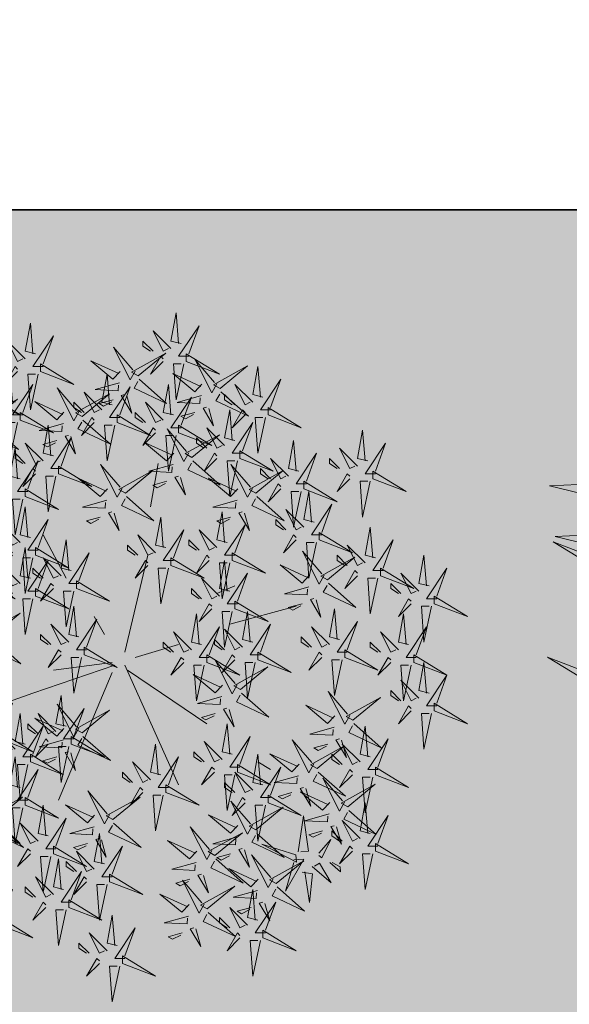
# Model space of a CAD drawing. Units: inches. Extents: x 1704 to 6393, y -157 to 1172.
# Tile 111 of 122: x 2667 to 2688, y 1003 to 1041. Entities that reach past the tile are written whole.
import ezdxf

# ---------------------------------------------------------------- set-up
doc = ezdxf.new("R2010")
doc.units = ezdxf.units.IN
doc.header["$MEASUREMENT"] = 0
for name, color, linetype, lineweight in [('A-ANNO-DIMS', 7, 'Continuous', 13), ('C-PROP', 7, 'Continuous', 35), ('L-shrub', 74, 'Continuous', 18)]:
    doc.layers.add(name, color=color, linetype=linetype, lineweight=lineweight)
doc.layers.add('L-HRDS-PATT', color=9, linetype='Continuous', lineweight=13, true_color=0xc5c1ba)
doc.styles.get("Standard").update_dxf_attribs({"font": 'arial.ttf'})
doc.dimstyles.get("Standard").update_dxf_attribs({"dimtxt": 6, "dimasz": 2, "dimexe": 0.18, "dimexo": 0.0625, "dimgap": 0.09, "dimtad": 0, "dimtih": 1, "dimtoh": 1, "dimdec": 1, "dimzin": 0, "dimdsep": 46, "dimlunit": 3, "dimtxsty": 'Standard', "dimblk": 'ARCHTICK', "dimcen": 0.09, "dimadec": 0, "dimazin": 0, "dimtfac": 1, "dimtdec": 1, "dimtofl": 0, "dimtmove": 0, "dimatfit": 3, "dimfxl": 1, "dimtolj": 1, "dimtzin": 0, "dimarcsym": 0})

# ---------------------------------------------------------------- blocks, each defined once
blk = doc.blocks.new('autumn shrub')
at = {"layer": 'L-shrub'}
for p, q in [((11.54, 1.92), (51.94, 98)), ((1.92, -3.84), (-38.48, 86.47)), ((-98.12, 69.17), (-107.74, 74.94)), ((0, 0), (-59.64, 40.35)), ((71.18, 17.29), (98.12, 26.9)), ((9.62, -3.84), (71.18, 17.29)), ((11.54, -5.76), (55.79, 0)), ((-5.77, -9.61), (-38.48, -19.21)), ((1.92, -13.45), (-15.39, -86.47)), ((17.31, -26.9), (25.01, -40.35)), ((-76.95, -34.59), (-126.97, -48.04)), ((-67.33, -57.64), (-80.8, -63.41)), ((46.17, -69.17), (63.49, -101.84)), ((-17.31, -122.97), (-23.09, -155.64))]:
    blk.add_line(p, q, dxfattribs=at)
for points in [[(5.77, 222.89), (11.54, 249.79), (13.47, 222.89), (7.7, 222.89)], [(-100.04, 203.68), (-94.27, 230.58), (-92.34, 203.68), (-98.12, 203.68)], [(3.85, 220.97), (-21.16, 230.58), (3.85, 215.21), (3.85, 220.97)], [(21.16, 220.97), (30.78, 230.58), (23.09, 217.13), (21.16, 219.05)], [(1.92, 217.13), (9.62, 217.13), (-5.77, 194.07), (1.92, 215.21)], [(98.12, 194.07), (103.89, 220.97), (105.81, 194.07), (100.04, 194.07)], [(-101.96, 201.75), (-126.97, 211.36), (-101.96, 195.99), (-101.96, 201.75)], [(-84.65, 201.75), (-75.03, 211.36), (-82.73, 197.91), (-84.65, 199.83)], [(-51.51, 194.97), (-55.15, 208.07), (-47.22, 194.76), (-49.84, 194.03)], [(15.39, 211.36), (28.86, 197.91), (21.16, 213.28), (17.31, 211.36)], [(28.86, 213.28), (36.55, 205.6), (36.55, 209.44), (30.78, 213.28)], [(-60.75, 182.51), (-81.34, 200.76), (-56.96, 189.22), (-59.8, 184.19)], [(-41.04, 197.9), (-30.56, 200.83), (-33.91, 202.71), (-40.09, 199.58)], [(7.7, 207.52), (15.39, 205.6), (11.54, 184.46), (9.62, 207.52)], [(46.17, 180.62), (51.94, 207.52), (53.87, 180.62), (48.1, 180.62)], [(96.19, 192.15), (71.18, 201.75), (96.19, 186.38), (96.19, 192.15)], [(113.51, 192.15), (123.13, 201.75), (115.43, 188.3), (113.51, 190.23)], [(-103.89, 197.91), (-96.19, 197.91), (-111.58, 174.85), (-103.89, 195.99)], [(-90.42, 192.15), (-76.95, 178.7), (-84.65, 194.07), (-88.5, 192.15)], [(-76.95, 194.07), (-69.26, 186.38), (-69.26, 190.23), (-75.03, 194.07)], [(-103.45, 175.76), (-107.1, 188.86), (-99.16, 175.55), (-101.78, 174.81)], [(-98.12, 188.3), (-90.42, 186.38), (-94.27, 165.25), (-96.19, 188.3)], [(-45.98, 185.23), (-27.65, 190.35), (-44.82, 191.2), (-45.03, 186.9)], [(15.39, 161.4), (21.16, 188.3), (23.09, 161.4), (17.31, 161.4)], [(44.25, 178.7), (19.24, 188.3), (44.25, 172.93), (44.25, 178.7)], [(61.56, 178.7), (71.18, 188.3), (63.49, 174.85), (61.56, 176.78)], [(94.27, 188.3), (101.96, 188.3), (86.57, 165.25), (94.27, 186.38)], [(-112.69, 163.3), (-133.28, 181.54), (-108.91, 170), (-111.74, 164.97)], [(-92.98, 178.69), (-82.5, 181.61), (-85.85, 183.5), (-92.03, 180.36)], [(-60.02, 179.89), (-80.67, 162.83), (-55, 177.06), (-60.02, 179.89)], [(-57.62, 176.33), (-53.83, 183.03), (-41.31, 158.3), (-55.94, 175.38)], [(-46.41, 176.64), (-40.96, 182.39), (-24.44, 168.66), (-45.47, 178.31)], [(100.04, 178.7), (107.74, 176.78), (103.89, 155.64), (101.96, 178.7)], [(107.74, 182.54), (121.2, 169.09), (113.51, 184.46), (109.66, 182.54)], [(121.2, 184.46), (128.9, 176.78), (128.9, 180.62), (123.13, 184.46)], [(138.52, 155.64), (144.29, 182.54), (146.21, 155.64), (140.44, 155.64)], [(-131.51, 152.18), (-139.33, 153.55), (-136.98, 174.91), (-133.43, 152.04)], [(-97.92, 166.01), (-79.59, 171.13), (-96.76, 171.98), (-96.98, 167.69)], [(42.32, 174.85), (50.02, 174.85), (34.63, 151.8), (42.32, 172.93)], [(55.79, 169.09), (69.26, 155.64), (61.56, 171.01), (57.72, 169.09)], [(69.26, 171.01), (76.95, 163.33), (76.95, 167.17), (71.18, 171.01)], [(-184.69, 138.35), (-178.92, 165.25), (-176.99, 138.35), (-182.77, 138.35)], [(-125.08, 143), (-132.76, 142.46), (-119.03, 166.55), (-125.21, 144.92)], [(-109.56, 157.11), (-105.78, 163.82), (-93.26, 139.08), (-107.89, 156.17)], [(-98.36, 157.42), (-92.9, 163.18), (-76.38, 149.44), (-97.41, 159.1)], [(-57.28, 154.62), (-60.92, 167.72), (-52.99, 154.41), (-55.61, 153.68)], [(13.47, 159.48), (-11.54, 169.09), (13.47, 153.72), (13.47, 159.48)], [(30.78, 159.48), (40.4, 169.09), (32.71, 155.64), (30.78, 157.56)], [(48.1, 165.25), (55.79, 163.33), (51.94, 142.19), (50.02, 165.25)], [(57.72, 140.27), (63.49, 167.17), (65.41, 140.27), (59.64, 140.27)], [(136.59, 153.72), (111.58, 163.33), (136.59, 147.95), (136.59, 153.72)], [(153.91, 153.72), (163.53, 163.33), (155.83, 149.87), (153.91, 151.8)], [(-138.92, 147.8), (-153.3, 160.27), (-144.54, 145.48), (-140.84, 147.67)], [(-111.96, 160.68), (-132.62, 143.61), (-106.94, 157.85), (-111.96, 160.68)], [(-66.52, 142.16), (-87.11, 160.4), (-62.74, 148.86), (-65.57, 143.84)], [(-46.81, 157.55), (-36.33, 160.48), (-39.68, 162.36), (-45.86, 159.22)], [(-152.22, 144.94), (-160.44, 152.06), (-160.16, 148.23), (-154.14, 144.8)], [(-88.06, 135.41), (-91.71, 148.51), (-83.77, 135.2), (-86.39, 134.46)], [(-51.75, 144.88), (-33.42, 150), (-50.59, 150.85), (-50.8, 146.55)], [(11.54, 155.64), (19.24, 155.64), (3.85, 132.58), (11.54, 153.72)], [(25.01, 149.87), (38.48, 136.42), (30.78, 151.8), (26.93, 149.87)], [(38.48, 151.8), (46.17, 144.11), (46.17, 147.95), (40.4, 151.8)], [(134.67, 149.87), (142.36, 149.87), (126.97, 126.82), (134.67, 147.95)], [(150.06, 122.97), (155.83, 149.87), (157.76, 122.97), (151.98, 122.97)], [(-186.61, 136.42), (-211.62, 146.03), (-186.61, 130.66), (-186.61, 136.42)], [(-169.3, 136.42), (-159.68, 146.03), (-167.38, 132.58), (-169.3, 134.5)], [(-144, 137.81), (-152.92, 127.55), (-146.19, 141.51), (-144.13, 139.73)], [(-126.73, 139.03), (-101.1, 131.22), (-127.13, 144.78), (-126.73, 139.03)], [(-97.3, 122.95), (-117.89, 141.19), (-93.52, 129.65), (-96.35, 124.62)], [(-77.59, 138.33), (-67.11, 141.26), (-70.46, 143.15), (-76.64, 140.01)], [(-63.39, 135.98), (-59.61, 142.68), (-47.08, 117.95), (-61.71, 135.03)], [(-52.18, 136.28), (-46.73, 142.04), (-30.21, 128.31), (-51.24, 137.96)], [(17.31, 146.03), (25.01, 144.11), (21.16, 122.97), (19.24, 146.03)], [(55.79, 138.35), (30.78, 147.95), (55.79, 132.58), (55.79, 138.35)], [(73.11, 138.35), (82.73, 147.95), (75.03, 134.5), (73.11, 136.42)], [(148.14, 144.11), (161.6, 130.66), (153.91, 146.03), (150.06, 144.11)], [(161.6, 146.03), (169.3, 138.35), (169.3, 142.19), (163.53, 146.03)], [(-128.51, 136.98), (-132.37, 109.74), (-136.19, 136.44), (-130.43, 136.85)], [(-65.79, 139.54), (-86.44, 122.48), (-60.77, 136.71), (-65.79, 139.54)], [(10.44, 115.26), (-10.16, 133.5), (14.22, 121.96), (11.38, 116.94)], [(19.67, 127.72), (16.03, 140.82), (23.96, 127.51), (21.35, 126.78)], [(30.15, 130.65), (40.62, 133.58), (37.28, 135.46), (31.09, 132.32)], [(53.87, 134.5), (61.56, 134.5), (46.17, 111.45), (53.87, 132.58)], [(98.93, 115.26), (78.34, 133.5), (102.71, 121.96), (99.88, 116.94)], [(108.17, 127.72), (104.53, 140.82), (112.46, 127.51), (109.84, 126.78)], [(118.64, 130.65), (129.12, 133.58), (125.77, 135.46), (119.59, 132.32)], [(140.44, 140.27), (148.14, 138.35), (144.29, 117.21), (142.36, 140.27)], [(-188.54, 132.58), (-180.84, 132.58), (-196.23, 109.52), (-188.54, 130.66)], [(-175.07, 126.82), (-161.6, 113.37), (-169.3, 128.74), (-173.15, 126.82)], [(-161.6, 128.74), (-153.91, 121.05), (-153.91, 124.9), (-159.68, 128.74)], [(-157.32, 118.11), (-160.96, 131.21), (-153.03, 117.9), (-155.65, 117.17)], [(-103.89, 101.84), (-98.12, 128.74), (-96.19, 101.84), (-101.96, 101.84)], [(-82.53, 125.66), (-64.2, 130.78), (-81.37, 131.63), (-81.59, 127.34)], [(67.33, 128.74), (80.8, 115.29), (73.11, 130.66), (69.26, 128.74)], [(78.88, 103.76), (84.65, 130.66), (86.57, 103.76), (80.8, 103.76)], [(80.8, 130.66), (88.5, 122.97), (88.5, 126.82), (82.73, 130.66)], [(148.14, 121.05), (123.13, 130.66), (148.14, 115.29), (148.14, 121.05)], [(165.45, 121.05), (175.07, 130.66), (167.38, 117.21), (165.45, 119.13)], [(-166.56, 105.65), (-187.15, 123.9), (-162.78, 112.36), (-165.61, 107.33)], [(-182.77, 122.97), (-175.07, 121.05), (-178.92, 99.92), (-180.84, 122.97)], [(-146.85, 121.04), (-136.37, 123.97), (-139.72, 125.86), (-145.9, 122.72)], [(-96.57, 120.33), (-117.23, 103.26), (-91.55, 117.49), (-96.57, 120.33)], [(-94.17, 116.76), (-90.39, 123.47), (-77.87, 98.73), (-92.49, 115.82)], [(-82.96, 117.07), (-77.51, 122.83), (-60.99, 109.09), (-82.02, 118.75)], [(-26.93, 94.15), (-21.16, 121.05), (-19.24, 94.15), (-25.01, 94.15)], [(25.2, 117.98), (43.54, 123.1), (26.37, 123.95), (26.15, 119.65)], [(59.64, 124.9), (67.33, 122.97), (63.49, 101.84), (61.56, 124.9)], [(113.7, 117.98), (132.03, 123.1), (114.86, 123.95), (114.65, 119.65)], [(200.08, 94.15), (205.85, 121.05), (207.78, 94.15), (202, 94.15)], [(-151.79, 108.37), (-133.46, 113.49), (-150.63, 114.34), (-150.84, 110.04)], [(11.17, 112.64), (-9.49, 95.58), (16.19, 109.81), (11.17, 112.64)], [(13.57, 109.08), (17.35, 115.78), (29.87, 91.05), (15.24, 108.13)], [(24.77, 109.38), (30.23, 115.14), (46.74, 101.41), (25.72, 111.06)], [(76.95, 101.84), (51.94, 111.45), (76.95, 96.07), (76.95, 101.84)], [(99.66, 112.64), (79.01, 95.58), (104.68, 109.81), (99.66, 112.64)], [(94.27, 101.84), (103.89, 111.45), (96.19, 98), (94.27, 99.92)], [(102.06, 109.08), (105.85, 115.78), (118.37, 91.05), (103.74, 108.13)], [(113.27, 109.38), (118.72, 115.14), (135.24, 101.41), (114.21, 111.06)], [(146.21, 117.21), (153.91, 117.21), (138.52, 94.15), (146.21, 115.29)], [(159.68, 111.45), (173.15, 98), (165.45, 113.37), (161.6, 111.45)], [(173.15, 113.37), (180.84, 105.68), (180.84, 109.52), (175.07, 113.37)], [(-184.69, 80.7), (-178.92, 107.6), (-176.99, 80.7), (-182.77, 80.7)], [(-163.43, 99.47), (-159.65, 106.17), (-147.12, 81.44), (-161.75, 98.53)], [(-152.22, 99.78), (-146.77, 105.54), (-130.25, 91.8), (-151.28, 101.45)], [(-105.81, 99.92), (-130.82, 109.52), (-105.81, 94.15), (-105.81, 99.92)], [(-88.5, 99.92), (-78.88, 109.52), (-86.57, 96.07), (-88.5, 98)], [(-80.8, 78.78), (-75.03, 105.68), (-73.11, 78.78), (-78.88, 78.78)], [(151.98, 107.6), (159.68, 105.68), (155.83, 84.54), (153.91, 107.6)], [(-165.83, 103.03), (-186.48, 85.97), (-160.81, 100.2), (-165.83, 103.03)], [(-134.24, 89.29), (-137.88, 102.39), (-129.94, 89.08), (-132.56, 88.35)], [(-123.76, 92.22), (-113.29, 95.15), (-116.63, 97.03), (-122.82, 93.89)], [(-28.86, 92.23), (-53.87, 101.84), (-28.86, 86.47), (-28.86, 92.23)], [(-11.54, 92.23), (-1.92, 101.84), (-9.62, 88.39), (-11.54, 90.31)], [(75.03, 98), (82.73, 98), (67.33, 74.94), (75.03, 96.07)], [(75.03, 71.09), (80.8, 98), (82.73, 71.09), (76.95, 71.09)], [(134.67, 76.86), (140.44, 103.76), (142.36, 76.86), (136.59, 76.86)], [(198.16, 92.23), (173.15, 101.84), (198.16, 86.47), (198.16, 92.23)], [(215.47, 92.23), (225.09, 101.84), (217.4, 88.39), (215.47, 90.31)], [(-143.47, 76.83), (-164.07, 95.07), (-139.69, 83.53), (-142.53, 78.51)], [(-107.74, 96.07), (-100.04, 96.07), (-115.43, 73.02), (-107.74, 94.15)], [(-94.27, 90.31), (-80.8, 76.86), (-88.5, 92.23), (-92.34, 90.31)], [(-80.8, 92.23), (-73.11, 84.54), (-73.11, 88.39), (-78.88, 92.23)], [(88.5, 92.23), (101.96, 78.78), (94.27, 94.15), (90.42, 92.23)], [(101.96, 94.15), (109.66, 86.47), (109.66, 90.31), (103.89, 94.15)], [(-186.61, 78.78), (-211.62, 88.39), (-186.61, 73.02), (-186.61, 78.78)], [(-169.3, 78.78), (-159.68, 88.39), (-167.38, 74.94), (-169.3, 76.86)], [(-128.7, 79.55), (-110.37, 84.67), (-127.54, 85.52), (-127.76, 81.22)], [(-82.73, 76.86), (-107.74, 86.47), (-82.73, 71.09), (-82.73, 76.86)], [(-101.96, 86.47), (-94.27, 84.54), (-98.12, 63.41), (-100.04, 86.47)], [(-65.41, 76.86), (-55.79, 86.47), (-63.49, 73.02), (-65.41, 74.94)], [(-30.78, 88.39), (-23.09, 88.39), (-38.48, 65.33), (-30.78, 86.47)], [(-17.31, 82.62), (-3.85, 69.17), (-11.54, 84.54), (-15.39, 82.62)], [(-3.85, 84.54), (3.85, 76.86), (3.85, 80.7), (-1.92, 84.54)], [(44.25, 57.64), (50.02, 84.54), (51.94, 57.64), (46.17, 57.64)], [(80.8, 88.39), (88.5, 86.47), (84.65, 65.33), (82.73, 88.39)], [(132.75, 74.94), (107.74, 84.54), (132.75, 69.17), (132.75, 74.94)], [(150.06, 74.94), (159.68, 84.54), (151.98, 71.09), (150.06, 73.02)], [(196.23, 88.39), (203.93, 88.39), (188.54, 65.33), (196.23, 86.47)], [(209.7, 82.62), (223.17, 69.17), (215.47, 84.54), (211.62, 82.62)], [(223.17, 84.54), (230.86, 76.86), (230.86, 80.7), (225.09, 84.54)], [(-188.54, 74.94), (-180.84, 74.94), (-196.23, 51.88), (-188.54, 73.02)], [(-142.74, 74.21), (-163.4, 57.15), (-137.72, 71.38), (-142.74, 74.21)], [(-140.34, 70.65), (-136.56, 77.35), (-124.04, 52.62), (-138.67, 69.7)], [(-129.14, 70.95), (-123.68, 76.71), (-107.16, 62.98), (-128.19, 72.63)], [(-25.01, 78.78), (-17.31, 76.86), (-21.16, 55.72), (-23.09, 78.78)], [(42.76, 62.39), (39.12, 75.49), (47.05, 62.18), (44.43, 61.45)], [(73.11, 69.17), (48.1, 78.78), (73.11, 63.41), (73.11, 69.17)], [(90.42, 69.17), (100.04, 78.78), (92.34, 65.33), (90.42, 67.25)], [(98.12, 53.8), (103.89, 80.7), (105.81, 53.8), (100.04, 53.8)], [(190.46, 53.8), (196.23, 80.7), (198.16, 53.8), (192.39, 53.8)], [(202, 78.78), (209.7, 76.86), (205.85, 55.72), (203.93, 78.78)], [(-175.07, 69.17), (-161.6, 55.72), (-169.3, 71.09), (-173.15, 69.17)], [(-161.6, 71.09), (-153.91, 63.41), (-153.91, 67.25), (-159.68, 71.09)], [(-84.65, 73.02), (-76.95, 73.02), (-92.34, 49.96), (-84.65, 71.09)], [(-71.18, 67.25), (-57.72, 53.8), (-65.41, 69.17), (-69.26, 67.25)], [(-57.72, 69.17), (-50.02, 61.49), (-50.02, 65.33), (-55.79, 69.17)], [(33.52, 49.93), (12.93, 68.17), (37.3, 56.63), (34.47, 51.61)], [(53.23, 65.32), (63.71, 68.25), (60.36, 70.13), (54.18, 66.99)], [(130.82, 71.09), (138.52, 71.09), (123.13, 48.04), (130.82, 69.17)], [(144.29, 65.33), (157.76, 51.88), (150.06, 67.25), (146.21, 65.33)], [(157.76, 67.25), (165.45, 59.57), (165.45, 63.41), (159.68, 67.25)], [(-228.94, 32.67), (-223.17, 59.57), (-221.24, 32.67), (-227.01, 32.67)], [(-182.77, 65.33), (-175.07, 63.41), (-178.92, 42.27), (-180.84, 65.33)], [(-161.17, 52.78), (-164.81, 65.88), (-156.88, 52.57), (-159.5, 51.84)], [(-150.69, 55.71), (-140.22, 58.64), (-143.57, 60.53), (-149.75, 57.39)], [(-78.88, 63.41), (-71.18, 61.49), (-75.03, 40.35), (-76.95, 63.41)], [(42.32, 55.72), (17.31, 65.33), (42.32, 49.96), (42.32, 55.72)], [(59.64, 55.72), (69.26, 65.33), (61.56, 51.88), (59.64, 53.8)], [(71.18, 65.33), (78.88, 65.33), (63.49, 42.27), (71.18, 63.41)], [(96.19, 51.88), (71.18, 61.49), (96.19, 46.12), (96.19, 51.88)], [(84.65, 59.57), (98.12, 46.12), (90.42, 61.49), (86.57, 59.57)], [(98.12, 61.49), (105.81, 53.8), (105.81, 57.64), (100.04, 61.49)], [(113.51, 51.88), (123.13, 61.49), (115.43, 48.04), (113.51, 49.96)], [(136.59, 61.49), (144.29, 59.57), (140.44, 38.43), (138.52, 61.49)], [(188.54, 51.88), (163.53, 61.49), (188.54, 46.12), (188.54, 51.88)], [(205.85, 51.88), (215.47, 61.49), (207.78, 48.04), (205.85, 49.96)], [(227.01, 32.67), (232.79, 59.57), (234.71, 32.67), (228.94, 32.67)], [(-170.4, 40.32), (-191, 58.57), (-166.62, 47.03), (-169.46, 42)], [(48.29, 52.64), (66.62, 57.77), (49.45, 58.62), (49.24, 54.32)], [(76.95, 55.72), (84.65, 53.8), (80.8, 32.67), (78.88, 55.72)], [(184.69, 30.74), (190.46, 57.64), (192.39, 30.74), (186.61, 30.74)], [(-155.64, 43.04), (-137.31, 48.16), (-154.48, 49.01), (-154.69, 44.71)], [(34.25, 47.31), (13.6, 30.25), (39.27, 44.48), (34.25, 47.31)], [(40.4, 51.88), (48.1, 51.88), (32.71, 28.82), (40.4, 49.96)], [(36.65, 43.75), (40.43, 50.45), (52.96, 25.72), (38.33, 42.8)], [(47.86, 44.05), (53.31, 49.81), (69.83, 36.08), (48.8, 45.73)], [(53.87, 46.12), (67.33, 32.67), (59.64, 48.04), (55.79, 46.12)], [(67.33, 48.04), (75.03, 40.35), (75.03, 44.19), (69.26, 48.04)], [(94.27, 48.04), (101.96, 48.04), (86.57, 24.98), (94.27, 46.12)], [(154.34, 31.65), (150.7, 44.75), (158.63, 31.44), (156.02, 30.7)], [(186.61, 48.04), (194.31, 48.04), (178.92, 24.98), (186.61, 46.12)], [(-230.86, 30.74), (-255.87, 40.35), (-230.86, 24.98), (-230.86, 30.74)], [(-213.55, 30.74), (-203.93, 40.35), (-211.62, 26.9), (-213.55, 28.82)], [(-169.68, 37.7), (-190.33, 20.64), (-164.66, 34.87), (-169.68, 37.7)], [(-167.27, 34.14), (-163.49, 40.84), (-150.97, 16.11), (-165.6, 33.2)], [(-156.07, 34.45), (-150.62, 40.21), (-134.1, 26.47), (-155.13, 36.12)], [(-76.52, 29.73), (-80.16, 42.83), (-72.23, 29.51), (-74.85, 28.78)], [(-66.05, 32.65), (-55.57, 35.58), (-58.92, 37.47), (-65.1, 34.33)], [(46.17, 42.27), (53.87, 40.35), (50.02, 19.21), (48.1, 42.27)], [(100.04, 38.43), (107.74, 36.51), (103.89, 15.37), (101.96, 38.43)], [(107.74, 42.27), (121.2, 28.82), (113.51, 44.19), (109.66, 42.27)], [(121.2, 44.19), (128.9, 36.51), (128.9, 40.35), (123.13, 44.19)], [(145.11, 19.19), (124.51, 37.43), (148.89, 25.89), (146.05, 20.86)], [(182.77, 28.82), (157.76, 38.43), (182.77, 23.06), (182.77, 28.82)], [(164.82, 34.57), (175.29, 37.5), (171.94, 39.39), (165.76, 36.25)], [(192.39, 38.43), (200.08, 36.51), (196.23, 15.37), (194.31, 38.43)], [(200.08, 42.27), (213.55, 28.82), (205.85, 44.19), (202, 42.27)], [(225.09, 30.74), (200.08, 40.35), (225.09, 24.98), (225.09, 30.74)], [(200.08, 28.82), (209.7, 38.43), (202, 24.98), (200.08, 26.9)], [(213.55, 44.19), (221.24, 36.51), (221.24, 40.35), (215.47, 44.19)], [(242.41, 30.74), (252.02, 40.35), (244.33, 26.9), (242.41, 28.82)], [(-85.76, 17.27), (-106.35, 35.51), (-81.97, 23.97), (-84.81, 18.94)], [(-232.79, 26.9), (-225.09, 26.9), (-240.48, 3.84), (-232.79, 24.98)], [(-219.32, 21.14), (-205.85, 7.69), (-213.55, 23.06), (-217.4, 21.14)], [(-213.55, -3.84), (-207.78, 23.06), (-205.85, -3.84), (-211.62, -3.84)], [(-205.85, 23.06), (-198.16, 15.37), (-198.16, 19.21), (-203.93, 23.06)], [(-70.99, 19.98), (-52.66, 25.1), (-69.83, 25.95), (-70.04, 21.66)], [(-57.72, -3.84), (-51.94, 23.06), (-50.02, -3.84), (-55.79, -3.84)], [(159.87, 21.9), (178.21, 27.02), (161.04, 27.87), (160.82, 23.58)], [(180.84, 24.98), (188.54, 24.98), (173.15, 1.92), (180.84, 23.06)], [(223.17, 26.9), (230.86, 26.9), (215.47, 3.84), (223.17, 24.98)], [(215.47, -1.92), (221.24, 24.98), (223.17, -1.92), (217.4, -1.92)], [(236.63, 21.14), (250.1, 7.69), (242.41, 23.06), (238.56, 21.14)], [(250.1, 23.06), (257.8, 15.37), (257.8, 19.21), (252.02, 23.06)], [(-227.01, 17.29), (-219.32, 15.37), (-223.17, -5.76), (-225.09, 17.29)], [(-161.6, -7.69), (-155.83, 19.21), (-153.91, -7.69), (-159.68, -7.69)], [(-96.19, -5.76), (-90.42, 21.14), (-88.5, -5.76), (-94.27, -5.76)], [(-82.63, 11.08), (-78.84, 17.78), (-66.32, -6.95), (-80.95, 10.14)], [(-71.42, 11.39), (-65.97, 17.15), (-49.45, 3.41), (-70.48, 13.06)], [(34.63, -9.61), (40.4, 17.29), (42.32, -9.61), (36.55, -9.61)], [(145.83, 16.57), (125.18, -0.5), (150.86, 13.74), (145.83, 16.57)], [(148.24, 13), (152.02, 19.71), (164.54, -5.03), (149.91, 12.06)], [(159.44, 13.31), (164.89, 19.07), (181.41, 5.33), (160.39, 14.99)], [(186.61, 15.37), (194.31, 13.45), (190.46, -7.69), (188.54, 15.37)], [(194.31, 19.21), (207.78, 5.76), (200.08, 21.14), (196.23, 19.21)], [(207.78, 21.14), (215.47, 13.45), (215.47, 17.29), (209.7, 21.14)], [(228.94, 17.29), (236.63, 15.37), (232.79, -5.76), (230.86, 17.29)], [(-85.03, 14.65), (-105.68, -2.42), (-80.01, 11.81), (-85.03, 14.65)], [(-215.47, -5.76), (-240.48, 3.84), (-215.47, -11.53), (-215.47, -5.76)], [(-198.16, -5.76), (-188.54, 3.84), (-196.23, -9.61), (-198.16, -7.69)], [(-163.53, -9.61), (-188.54, 0), (-163.53, -15.37), (-163.53, -9.61)], [(-146.21, -9.61), (-136.59, 0), (-144.29, -13.45), (-146.21, -11.53)], [(-98.12, -7.69), (-123.13, 1.92), (-98.12, -13.45), (-98.12, -7.69)], [(-59.64, -5.76), (-84.65, 3.84), (-59.64, -11.53), (-59.64, -5.76)], [(-80.8, -7.69), (-71.18, 1.92), (-78.88, -11.53), (-80.8, -9.61)], [(-42.32, -5.76), (-32.71, 3.84), (-40.4, -9.61), (-42.32, -7.69)], [(110.09, -10.62), (106.45, 2.47), (114.39, -10.84), (111.77, -11.57)], [(213.55, -3.84), (188.54, 5.76), (213.55, -9.61), (213.55, -3.84)], [(230.86, -3.84), (240.48, 5.76), (232.79, -7.69), (230.86, -5.76)], [(232.79, -26.9), (238.56, 0), (240.48, -26.9), (234.71, -26.9)], [(32.71, -11.53), (7.7, -1.92), (32.71, -17.29), (32.71, -11.53)], [(50.02, -11.53), (59.64, -1.92), (51.94, -15.37), (50.02, -13.45)], [(100.86, -23.09), (80.26, -4.84), (104.64, -16.38), (101.8, -21.41)], [(120.57, -7.7), (131.04, -4.77), (127.7, -2.88), (121.51, -6.02)], [(-217.4, -9.61), (-209.7, -9.61), (-225.09, -32.67), (-217.4, -11.53)], [(-203.93, -15.37), (-190.46, -28.82), (-198.16, -13.45), (-202, -15.37)], [(-190.46, -13.45), (-182.77, -21.14), (-182.77, -17.29), (-188.54, -13.45)], [(-165.45, -13.45), (-157.76, -13.45), (-173.15, -36.51), (-165.45, -15.37)], [(-100.04, -11.53), (-92.34, -11.53), (-107.74, -34.59), (-100.04, -13.45)], [(-61.56, -9.61), (-53.87, -9.61), (-69.26, -32.67), (-61.56, -11.53)], [(-48.1, -15.37), (-34.63, -28.82), (-42.32, -13.45), (-46.17, -15.37)], [(-34.63, -13.45), (-26.93, -21.14), (-26.93, -17.29), (-32.71, -13.45)], [(115.63, -20.37), (133.96, -15.25), (116.79, -14.4), (116.57, -18.7)], [(211.62, -7.69), (219.32, -7.69), (203.93, -30.74), (211.62, -9.61)], [(225.09, -13.45), (238.56, -26.9), (230.86, -11.53), (227.01, -13.45)], [(238.56, -11.53), (246.25, -19.21), (246.25, -15.37), (240.48, -11.53)], [(-228.94, -48.04), (-223.17, -21.14), (-221.24, -48.04), (-227.01, -48.04)], [(-211.62, -19.21), (-203.93, -21.14), (-207.78, -42.27), (-209.7, -19.21)], [(-151.98, -19.21), (-138.52, -32.67), (-146.21, -17.29), (-150.06, -19.21)], [(-138.52, -17.29), (-130.82, -24.98), (-130.82, -21.14), (-136.59, -17.29)], [(-94.27, -21.14), (-86.57, -23.06), (-90.42, -44.19), (-92.34, -21.14)], [(-86.57, -17.29), (-73.11, -30.74), (-80.8, -15.37), (-84.65, -17.29)], [(-78.88, -44.19), (-73.11, -17.29), (-71.18, -44.19), (-76.95, -44.19)], [(-73.11, -15.37), (-65.41, -23.06), (-65.41, -19.21), (-71.18, -15.37)], [(-55.79, -19.21), (-48.1, -21.14), (-51.94, -42.27), (-53.87, -19.21)], [(30.78, -15.37), (38.48, -15.37), (23.09, -38.43), (30.78, -17.29)], [(44.25, -21.14), (57.72, -34.59), (50.02, -19.21), (46.17, -21.14)], [(57.72, -19.21), (65.41, -26.9), (65.41, -23.06), (59.64, -19.21)], [(230.86, -28.82), (205.85, -19.21), (230.86, -34.59), (230.86, -28.82)], [(217.4, -17.29), (225.09, -19.21), (221.24, -40.35), (219.32, -17.29)], [(248.18, -28.82), (257.8, -19.21), (250.1, -32.67), (248.18, -30.74)], [(-159.68, -23.06), (-151.98, -24.98), (-155.83, -46.12), (-157.76, -23.06)], [(36.55, -24.98), (44.25, -26.9), (40.4, -48.04), (38.48, -24.98)], [(71.18, -53.8), (76.95, -26.9), (78.88, -53.8), (73.11, -53.8)], [(101.59, -25.71), (80.93, -42.77), (106.61, -28.54), (101.59, -25.71)], [(103.99, -29.27), (107.77, -22.57), (120.29, -47.3), (105.66, -30.21)], [(115.19, -28.96), (120.65, -23.2), (137.17, -36.94), (116.14, -27.29)], [(173.15, -55.72), (178.92, -28.82), (180.84, -55.72), (175.07, -55.72)], [(-80.8, -46.12), (-105.81, -36.51), (-80.8, -51.88), (-80.8, -46.12)], [(-63.49, -46.12), (-53.87, -36.51), (-61.56, -49.96), (-63.49, -48.04)], [(40.4, -59.57), (46.17, -32.67), (48.1, -59.57), (42.32, -59.57)], [(111.58, -61.49), (117.35, -34.59), (119.28, -61.49), (113.51, -61.49)], [(228.94, -32.67), (236.63, -32.67), (221.24, -55.72), (228.94, -34.59)], [(242.41, -38.43), (255.87, -51.88), (248.18, -36.51), (244.33, -38.43)], [(255.87, -36.51), (263.57, -44.19), (263.57, -40.35), (257.8, -36.51)], [(-230.86, -49.96), (-255.87, -40.35), (-230.86, -55.72), (-230.86, -49.96)], [(-213.55, -49.96), (-203.93, -40.35), (-211.62, -53.8), (-213.55, -51.88)], [(-188.54, -69.17), (-182.77, -42.27), (-180.84, -69.17), (-186.61, -69.17)], [(-141.93, -52.9), (-145.57, -39.8), (-137.64, -53.11), (-140.26, -53.84)], [(234.71, -42.27), (242.41, -44.19), (238.56, -65.33), (236.63, -42.27)], [(-151.17, -65.36), (-171.76, -47.11), (-147.39, -58.66), (-150.22, -63.68)], [(-131.46, -49.97), (-120.98, -47.04), (-124.33, -45.16), (-130.51, -48.29)], [(-82.73, -49.96), (-75.03, -49.96), (-90.42, -73.02), (-82.73, -51.88)], [(-30.78, -76.86), (-25.01, -49.96), (-23.09, -76.86), (-28.86, -76.86)], [(38.48, -61.49), (13.47, -51.88), (38.48, -67.25), (38.48, -61.49)], [(69.26, -55.72), (44.25, -46.12), (69.26, -61.49), (69.26, -55.72)], [(55.79, -61.49), (65.41, -51.88), (57.72, -65.33), (55.79, -63.41)], [(86.57, -55.72), (96.19, -46.12), (88.5, -59.57), (86.57, -57.64)], [(171.22, -57.64), (146.21, -48.04), (171.22, -63.41), (171.22, -57.64)], [(188.54, -57.64), (198.16, -48.04), (190.46, -61.49), (188.54, -59.57)], [(-232.79, -53.8), (-225.09, -53.8), (-240.48, -76.86), (-232.79, -55.72)], [(-219.32, -59.57), (-205.85, -73.02), (-213.55, -57.64), (-217.4, -59.57)], [(-205.85, -57.64), (-198.16, -65.33), (-198.16, -61.49), (-203.93, -57.64)], [(-136.4, -62.64), (-118.07, -57.52), (-135.24, -56.67), (-135.45, -60.97)], [(-76.95, -80.7), (-71.18, -53.8), (-69.26, -80.7), (-75.03, -80.7)], [(-69.26, -55.72), (-55.79, -69.17), (-63.49, -53.8), (-67.33, -55.72)], [(-55.79, -53.8), (-48.1, -61.49), (-48.1, -57.64), (-53.87, -53.8)], [(71.18, -84.54), (76.95, -57.64), (78.88, -84.54), (73.11, -84.54)], [(109.66, -63.41), (84.65, -53.8), (109.66, -69.17), (109.66, -63.41)], [(126.97, -63.41), (136.59, -53.8), (128.9, -67.25), (126.97, -65.33)], [(211.62, -82.62), (217.4, -55.72), (219.32, -82.62), (213.55, -82.62)], [(-227.01, -63.41), (-219.32, -65.33), (-223.17, -86.47), (-225.09, -63.41)], [(-190.46, -71.09), (-215.47, -61.49), (-190.46, -76.86), (-190.46, -71.09)], [(-173.15, -71.09), (-163.53, -61.49), (-171.22, -74.94), (-173.15, -73.02)], [(-148.04, -71.54), (-144.26, -64.84), (-131.73, -89.57), (-146.36, -72.49)], [(-136.83, -71.23), (-131.38, -65.48), (-114.86, -79.21), (-135.89, -69.56)], [(-76.95, -59.57), (-69.26, -61.49), (-73.11, -82.62), (-75.03, -59.57)], [(36.55, -65.33), (44.25, -65.33), (28.86, -88.39), (36.55, -67.25)], [(67.33, -59.57), (75.03, -59.57), (59.64, -82.62), (67.33, -61.49)], [(80.8, -65.33), (94.27, -78.78), (86.57, -63.41), (82.73, -65.33)], [(94.27, -63.41), (101.96, -71.09), (101.96, -67.25), (96.19, -63.41)], [(150.49, -79.8), (146.85, -66.7), (154.79, -80.01), (152.17, -80.74)], [(169.3, -61.49), (176.99, -61.49), (161.6, -84.54), (169.3, -63.41)], [(182.77, -67.25), (196.23, -80.7), (188.54, -65.33), (184.69, -67.25)], [(196.23, -65.33), (203.93, -73.02), (203.93, -69.17), (198.16, -65.33)], [(-150.44, -67.98), (-171.09, -85.04), (-145.42, -70.81), (-150.44, -67.98)], [(-142.36, -96.07), (-136.59, -69.17), (-134.67, -96.07), (-140.44, -96.07)], [(-78.88, -82.62), (-103.89, -73.02), (-78.88, -88.39), (-78.88, -82.62)], [(-61.56, -82.62), (-51.94, -73.02), (-59.64, -86.47), (-61.56, -84.54)], [(-32.71, -78.78), (-57.72, -69.17), (-32.71, -84.54), (-32.71, -78.78)], [(-15.39, -78.78), (-5.77, -69.17), (-13.47, -82.62), (-15.39, -80.7)], [(50.02, -71.09), (63.49, -84.54), (55.79, -69.17), (51.94, -71.09)], [(63.49, -69.17), (71.18, -76.86), (71.18, -73.02), (65.41, -69.17)], [(73.11, -69.17), (80.8, -71.09), (76.95, -92.23), (75.03, -69.17)], [(107.74, -67.25), (115.43, -67.25), (100.04, -90.31), (107.74, -69.17)], [(141.26, -92.26), (120.66, -74.02), (145.04, -85.56), (142.2, -90.58)], [(121.2, -73.02), (134.67, -86.47), (126.97, -71.09), (123.13, -73.02)], [(134.67, -71.09), (142.36, -78.78), (142.36, -74.94), (136.59, -71.09)], [(160.97, -76.87), (171.44, -73.94), (168.1, -72.06), (161.91, -75.19)], [(175.07, -71.09), (182.77, -73.02), (178.92, -94.15), (176.99, -71.09)], [(-192.39, -74.94), (-184.69, -74.94), (-200.08, -98), (-192.39, -76.86)], [(-178.92, -80.7), (-165.45, -94.15), (-173.15, -78.78), (-176.99, -80.7)], [(-165.45, -78.78), (-157.76, -86.47), (-157.76, -82.62), (-163.53, -78.78)], [(42.32, -74.94), (50.02, -76.86), (46.17, -98), (44.25, -74.94)], [(69.26, -86.47), (44.25, -76.86), (69.26, -92.23), (69.26, -86.47)], [(86.57, -86.47), (96.19, -76.86), (88.5, -90.31), (86.57, -88.39)], [(113.51, -76.86), (121.2, -78.78), (117.35, -99.92), (115.43, -76.86)], [(209.7, -84.54), (184.69, -74.94), (209.7, -90.31), (209.7, -84.54)], [(227.01, -84.54), (236.63, -74.94), (228.94, -88.39), (227.01, -86.47)], [(-186.61, -84.54), (-178.92, -86.47), (-182.77, -107.6), (-184.69, -84.54)], [(-144.29, -98), (-169.3, -88.39), (-144.29, -103.76), (-144.29, -98)], [(-126.97, -98), (-117.35, -88.39), (-125.05, -101.84), (-126.97, -99.92)], [(-80.8, -86.47), (-73.11, -86.47), (-88.5, -109.52), (-80.8, -88.39)], [(-34.63, -82.62), (-26.93, -82.62), (-42.32, -105.68), (-34.63, -84.54)], [(-21.16, -88.39), (-7.7, -101.84), (-15.39, -86.47), (-19.24, -88.39)], [(-7.7, -86.47), (0, -94.15), (0, -90.31), (-5.77, -86.47)], [(156.03, -89.54), (174.36, -84.42), (157.19, -83.57), (156.97, -87.87)], [(186.61, -115.29), (192.39, -88.39), (194.31, -115.29), (188.54, -115.29)], [(207.78, -88.39), (215.47, -88.39), (200.08, -111.45), (207.78, -90.31)], [(-75.03, -96.07), (-67.33, -98), (-71.18, -119.13), (-73.11, -96.07)], [(-67.33, -92.23), (-53.87, -105.68), (-61.56, -90.31), (-65.41, -92.23)], [(-53.87, -90.31), (-46.17, -98), (-46.17, -94.15), (-51.94, -90.31)], [(-28.86, -92.23), (-21.16, -94.15), (-25.01, -115.29), (-26.93, -92.23)], [(67.33, -90.31), (75.03, -90.31), (59.64, -113.37), (67.33, -92.23)], [(80.8, -96.07), (94.27, -109.52), (86.57, -94.15), (82.73, -96.07)], [(94.27, -94.15), (101.96, -101.84), (101.96, -98), (96.19, -94.15)], [(141.99, -94.88), (121.33, -111.94), (147.01, -97.71), (141.99, -94.88)], [(144.39, -98.44), (148.17, -91.74), (160.69, -116.47), (146.06, -99.39)], [(155.59, -98.13), (161.05, -92.38), (177.57, -106.11), (156.54, -96.46)], [(221.24, -94.15), (234.71, -107.6), (227.01, -92.23), (223.17, -94.15)], [(234.71, -92.23), (242.41, -99.92), (242.41, -96.07), (236.63, -92.23)], [(-146.21, -101.84), (-138.52, -101.84), (-153.91, -124.9), (-146.21, -103.76)], [(73.11, -99.92), (80.8, -101.84), (76.95, -122.97), (75.03, -99.92)], [(78.88, -128.74), (84.65, -101.84), (86.57, -128.74), (80.8, -128.74)], [(213.55, -98), (221.24, -99.92), (217.4, -121.05), (215.47, -98)], [(-132.75, -107.6), (-119.28, -121.05), (-126.97, -105.68), (-130.82, -107.6)], [(-130.82, -134.5), (-125.05, -107.6), (-123.13, -134.5), (-128.9, -134.5)], [(-119.28, -105.68), (-111.58, -113.37), (-111.58, -109.52), (-117.35, -105.68)], [(-88.06, -118.23), (-91.71, -105.13), (-83.77, -118.44), (-86.39, -119.17)], [(-77.59, -115.3), (-67.11, -112.37), (-70.46, -110.49), (-76.64, -113.62)], [(10.05, -118.23), (6.41, -105.13), (14.35, -118.44), (11.73, -119.17)], [(20.53, -115.3), (31, -112.37), (27.66, -110.49), (21.47, -113.62)], [(184.69, -117.21), (159.68, -107.6), (184.69, -122.97), (184.69, -117.21)], [(202, -117.21), (211.62, -107.6), (203.93, -121.05), (202, -119.13)], [(-182.77, -142.19), (-176.99, -115.29), (-175.07, -142.19), (-180.84, -142.19)], [(-140.44, -111.45), (-132.75, -113.37), (-136.59, -134.5), (-138.52, -111.45)], [(-97.3, -130.69), (-117.89, -112.44), (-93.52, -123.99), (-96.35, -129.01)], [(0.82, -130.69), (-19.78, -112.44), (4.6, -123.99), (1.76, -129.01)], [(127.41, -125.91), (123.77, -112.81), (131.7, -126.12), (129.08, -126.86)], [(137.88, -122.99), (148.36, -120.06), (145.01, -118.17), (138.83, -121.31)], [(-82.53, -127.97), (-64.2, -122.85), (-81.37, -122), (-81.59, -126.3)], [(15.59, -127.97), (33.92, -122.85), (16.75, -122), (16.53, -126.3)], [(76.95, -130.66), (51.94, -121.05), (76.95, -136.42), (76.95, -130.66)], [(53.87, -146.03), (59.64, -119.13), (61.56, -146.03), (55.79, -146.03)], [(94.27, -130.66), (103.89, -121.05), (96.19, -134.5), (94.27, -132.58)], [(118.17, -138.37), (97.58, -120.13), (121.95, -131.67), (119.12, -136.7)], [(163.53, -146.03), (169.3, -119.13), (171.22, -146.03), (165.45, -146.03)], [(182.77, -121.05), (190.46, -121.05), (175.07, -144.11), (182.77, -122.97)], [(196.23, -126.82), (209.7, -140.27), (202, -124.9), (198.16, -126.82)], [(209.7, -124.9), (217.4, -132.58), (217.4, -128.74), (211.62, -124.9)], [(-132.75, -136.42), (-157.76, -126.82), (-132.75, -142.19), (-132.75, -136.42)], [(-96.57, -133.31), (-117.23, -150.37), (-91.55, -136.14), (-96.57, -133.31)], [(-115.43, -136.42), (-105.81, -126.82), (-113.51, -140.27), (-115.43, -138.35)], [(-94.17, -136.87), (-90.39, -130.17), (-77.87, -154.9), (-92.49, -137.82)], [(-82.96, -136.56), (-77.51, -130.81), (-60.99, -144.54), (-82.02, -134.89)], [(-82.73, -157.56), (-76.95, -130.66), (-75.03, -157.56), (-80.8, -157.56)], [(-39.97, -145.13), (-43.61, -132.03), (-35.67, -145.34), (-38.29, -146.07)], [(1.55, -133.31), (-19.11, -150.37), (6.57, -136.14), (1.55, -133.31)], [(3.95, -136.87), (7.73, -130.17), (20.25, -154.9), (5.62, -137.82)], [(15.15, -136.56), (20.61, -130.81), (37.13, -144.54), (16.1, -134.89)], [(132.94, -135.66), (151.27, -130.54), (134.1, -129.69), (133.89, -133.98)], [(188.54, -130.66), (196.23, -132.58), (192.39, -153.72), (190.46, -130.66)], [(-184.69, -144.11), (-209.7, -134.5), (-184.69, -149.87), (-184.69, -144.11)], [(-167.38, -144.11), (-157.76, -134.5), (-165.45, -147.95), (-167.38, -146.03)], [(-134.67, -140.27), (-126.97, -140.27), (-142.36, -163.33), (-134.67, -142.19)], [(-49.2, -157.59), (-69.8, -139.35), (-45.42, -150.89), (-48.26, -155.91)], [(-29.49, -142.2), (-19.02, -139.27), (-22.36, -137.39), (-28.55, -140.52)], [(51.94, -147.95), (26.93, -138.35), (51.94, -153.72), (51.94, -147.95)], [(75.03, -134.5), (82.73, -134.5), (67.33, -157.56), (75.03, -136.42)], [(69.26, -147.95), (78.88, -138.35), (71.18, -151.8), (69.26, -149.87)], [(88.5, -140.27), (101.96, -153.72), (94.27, -138.35), (90.42, -140.27)], [(101.96, -138.35), (109.66, -146.03), (109.66, -142.19), (103.89, -138.35)], [(121.3, -144.56), (125.08, -137.85), (137.61, -162.59), (122.98, -145.5)], [(132.51, -144.25), (137.96, -138.49), (154.48, -152.23), (133.45, -142.57)], [(161.6, -147.95), (136.59, -138.35), (161.6, -153.72), (161.6, -147.95)], [(178.92, -147.95), (188.54, -138.35), (180.84, -151.8), (178.92, -149.87)], [(-186.61, -147.95), (-178.92, -147.95), (-194.31, -171.01), (-186.61, -149.87)], [(-121.2, -146.03), (-107.74, -159.48), (-115.43, -144.11), (-119.28, -146.03)], [(-107.74, -144.11), (-100.04, -151.8), (-100.04, -147.95), (-105.81, -144.11)], [(80.8, -144.11), (88.5, -146.03), (84.65, -167.17), (82.73, -144.11)], [(118.9, -140.99), (98.25, -158.06), (123.92, -143.83), (118.9, -140.99)], [(-173.15, -153.72), (-159.68, -167.17), (-167.38, -151.8), (-171.22, -153.72)], [(-159.68, -151.8), (-151.98, -159.48), (-151.98, -155.64), (-157.76, -151.8)], [(-128.9, -149.87), (-121.2, -151.8), (-125.05, -172.93), (-126.97, -149.87)], [(-84.65, -159.48), (-109.66, -149.87), (-84.65, -165.25), (-84.65, -159.48)], [(-67.33, -159.48), (-57.72, -149.87), (-65.41, -163.33), (-67.33, -161.4)], [(-36.55, -176.78), (-30.78, -149.87), (-28.86, -176.78), (-34.63, -176.78)], [(-34.43, -154.87), (-16.1, -149.75), (-33.27, -148.9), (-33.49, -153.2)], [(50.02, -151.8), (57.72, -151.8), (42.32, -174.85), (50.02, -153.72)], [(63.49, -157.56), (76.95, -171.01), (69.26, -155.64), (65.41, -157.56)], [(76.95, -155.64), (84.65, -163.33), (84.65, -159.48), (78.88, -155.64)], [(159.68, -151.8), (167.38, -151.8), (151.98, -174.85), (159.68, -153.72)], [(173.15, -157.56), (186.61, -171.01), (178.92, -155.64), (175.07, -157.56)], [(186.61, -155.64), (194.31, -163.33), (194.31, -159.48), (188.54, -155.64)], [(-180.84, -157.56), (-173.15, -159.48), (-176.99, -180.62), (-178.92, -157.56)], [(-48.47, -160.21), (-69.13, -177.27), (-43.45, -163.04), (-48.47, -160.21)], [(-46.07, -163.77), (-42.29, -157.07), (-29.77, -181.8), (-44.4, -164.72)], [(-34.87, -163.46), (-29.41, -157.71), (-12.89, -171.44), (-33.92, -161.79)], [(9.62, -184.46), (15.39, -157.56), (17.31, -184.46), (11.54, -184.46)], [(42.76, -175.87), (39.12, -162.77), (47.05, -176.08), (44.43, -176.81)], [(55.79, -161.4), (63.49, -163.33), (59.64, -184.46), (57.72, -161.4)], [(82.73, -186.38), (88.5, -159.48), (90.42, -186.38), (84.65, -186.38)], [(112.02, -172.03), (108.37, -158.93), (116.31, -172.24), (113.69, -172.97)], [(165.45, -161.4), (173.15, -163.33), (169.3, -184.46), (167.38, -161.4)], [(-103.89, -190.23), (-98.12, -163.33), (-96.19, -190.23), (-101.96, -190.23)], [(-86.57, -163.33), (-78.88, -163.33), (-94.27, -186.38), (-86.57, -165.25)], [(-73.11, -169.09), (-59.64, -182.54), (-67.33, -167.17), (-71.18, -169.09)], [(-38.48, -178.7), (-63.49, -169.09), (-38.48, -184.46), (-38.48, -178.7)], [(-59.64, -167.17), (-51.94, -174.85), (-51.94, -171.01), (-57.72, -167.17)], [(-21.16, -178.7), (-11.54, -169.09), (-19.24, -182.54), (-21.16, -180.62)], [(33.52, -188.33), (12.93, -170.09), (37.3, -181.63), (34.47, -186.66)], [(53.23, -172.94), (63.71, -170.02), (60.36, -168.13), (54.18, -171.27)], [(102.78, -184.49), (82.19, -166.25), (106.56, -177.79), (103.73, -182.81)], [(122.49, -169.1), (132.97, -166.17), (129.62, -164.29), (123.44, -167.43)], [(-80.8, -172.93), (-73.11, -174.85), (-76.95, -195.99), (-78.88, -172.93)], [(7.7, -186.38), (-17.31, -176.78), (7.7, -192.15), (7.7, -186.38)], [(25.01, -186.38), (34.63, -176.78), (26.93, -190.23), (25.01, -188.3)], [(107.74, -199.83), (113.51, -172.93), (115.43, -199.83), (109.66, -199.83)], [(117.55, -181.77), (135.88, -176.65), (118.71, -175.8), (118.49, -180.1)], [(-105.81, -192.15), (-130.82, -182.54), (-105.81, -197.91), (-105.81, -192.15)], [(-88.5, -192.15), (-78.88, -182.54), (-86.57, -195.99), (-88.5, -194.07)], [(-61.13, -197.01), (-64.77, -183.91), (-56.84, -197.22), (-59.46, -197.95)], [(-40.4, -182.54), (-32.71, -182.54), (-48.1, -205.6), (-40.4, -184.46)], [(48.29, -185.62), (66.62, -180.5), (49.45, -179.65), (49.24, -183.94)], [(80.8, -188.3), (55.79, -178.7), (80.8, -194.07), (80.8, -188.3)], [(98.12, -188.3), (107.74, -178.7), (100.04, -192.15), (98.12, -190.23)], [(105.91, -190.67), (109.69, -183.97), (122.21, -208.7), (107.59, -191.62)], [(117.12, -190.37), (122.57, -184.61), (139.09, -198.34), (118.06, -188.69)], [(-70.36, -209.47), (-90.96, -191.23), (-66.58, -202.77), (-69.42, -207.79)], [(-50.65, -194.08), (-40.18, -191.15), (-43.53, -189.27), (-49.71, -192.4)], [(-34.63, -192.15), (-26.93, -194.07), (-30.78, -215.21), (-32.71, -192.15)], [(-26.93, -188.3), (-13.47, -201.75), (-21.16, -186.38), (-25.01, -188.3)], [(-13.47, -186.38), (-5.77, -194.07), (-5.77, -190.23), (-11.54, -186.38)], [(5.77, -190.23), (13.47, -190.23), (-1.92, -213.28), (5.77, -192.15)], [(34.25, -190.95), (13.6, -208.02), (39.27, -193.78), (34.25, -190.95)], [(36.65, -194.52), (40.43, -187.81), (52.96, -212.55), (38.33, -195.46)], [(47.86, -194.21), (53.31, -188.45), (69.83, -202.19), (48.8, -192.53)], [(78.88, -192.15), (86.57, -192.15), (71.18, -215.21), (78.88, -194.07)], [(105.81, -201.75), (80.8, -192.15), (105.81, -207.52), (105.81, -201.75)], [(103.51, -187.11), (82.85, -204.17), (108.53, -189.94), (103.51, -187.11)], [(123.13, -201.75), (132.75, -192.15), (125.05, -205.6), (123.13, -203.68)], [(-107.74, -195.99), (-100.04, -195.99), (-115.43, -219.05), (-107.74, -197.91)], [(-94.27, -201.75), (-80.8, -215.21), (-88.5, -199.83), (-92.34, -201.75)], [(-80.8, -199.83), (-73.11, -207.52), (-73.11, -203.68), (-78.88, -199.83)], [(0.43, -206.61), (-3.21, -193.52), (4.73, -206.83), (2.11, -207.56)], [(10.91, -203.69), (21.38, -200.76), (18.04, -198.87), (11.85, -202.01)], [(11.54, -199.83), (19.24, -201.75), (15.39, -222.89), (13.47, -199.83)], [(19.24, -195.99), (32.71, -209.44), (25.01, -194.07), (21.16, -195.99)], [(32.71, -194.07), (40.4, -201.75), (40.4, -197.91), (34.63, -194.07)], [(67.33, -222.89), (73.11, -195.99), (75.03, -222.89), (69.26, -222.89)], [(92.34, -197.91), (105.81, -211.36), (98.12, -195.99), (94.27, -197.91)], [(105.81, -195.99), (113.51, -203.68), (113.51, -199.83), (107.74, -195.99)], [(-101.96, -205.6), (-94.27, -207.52), (-98.12, -228.66), (-100.04, -205.6)], [(-55.6, -206.75), (-37.27, -201.63), (-54.44, -200.78), (-54.65, -205.08)], [(-42.32, -230.58), (-36.55, -203.68), (-34.63, -230.58), (-40.4, -230.58)], [(-8.8, -219.08), (-29.4, -200.83), (-5.02, -212.37), (-7.86, -217.4)], [(84.65, -201.75), (92.34, -203.68), (88.5, -224.81), (86.57, -201.75)], [(103.89, -205.6), (111.58, -205.6), (96.19, -228.66), (103.89, -207.52)], [(-69.64, -212.09), (-90.29, -229.15), (-64.62, -214.92), (-69.64, -212.09)], [(-67.23, -215.65), (-63.45, -208.95), (-50.93, -233.68), (-65.56, -216.6)], [(-56.03, -215.34), (-50.58, -209.59), (-34.06, -223.32), (-55.09, -213.67)], [(5.97, -216.36), (24.3, -211.24), (7.13, -210.39), (6.91, -214.69)], [(117.35, -211.36), (130.82, -224.81), (123.13, -209.44), (119.28, -211.36)], [(130.82, -209.44), (138.52, -217.13), (138.52, -213.28), (132.75, -209.44)], [(-8.07, -221.7), (-28.73, -238.76), (-3.05, -224.53), (-8.07, -221.7)], [(-5.67, -225.26), (-1.89, -218.56), (10.63, -243.29), (-4, -226.2)], [(5.53, -224.95), (10.99, -219.19), (27.51, -232.93), (6.48, -223.28)], [(65.41, -224.81), (40.4, -215.21), (65.41, -230.58), (65.41, -224.81)], [(82.73, -224.81), (92.34, -215.21), (84.65, -228.66), (82.73, -226.73)], [(109.66, -215.21), (117.35, -217.13), (113.51, -238.26), (111.58, -215.21)], [(-44.25, -232.5), (-69.26, -222.89), (-44.25, -238.26), (-44.25, -232.5)], [(-26.93, -232.5), (-17.31, -222.89), (-25.01, -236.34), (-26.93, -234.42)], [(63.49, -228.66), (71.18, -228.66), (55.79, -251.71), (63.49, -230.58)], [(-46.17, -236.34), (-38.48, -236.34), (-53.87, -259.4), (-46.17, -238.26)], [(76.95, -234.42), (90.42, -247.87), (82.73, -232.5), (78.88, -234.42)], [(90.42, -232.5), (98.12, -240.18), (98.12, -236.34), (92.34, -232.5)], [(-32.71, -242.11), (-19.24, -255.56), (-26.93, -240.18), (-30.78, -242.11)], [(-19.24, -240.18), (-11.54, -247.87), (-11.54, -244.03), (-17.31, -240.18)], [(69.26, -238.26), (76.95, -240.18), (73.11, -261.32), (71.18, -238.26)], [(-40.4, -245.95), (-32.71, -247.87), (-36.55, -269.01), (-38.48, -245.95)]]:
    blk.add_lwpolyline(points, dxfattribs=at)
blk = doc.blocks.new('shrub3')
for points in [[(277.74, 36.65), (307.75, 25.12), (277.74, 43.57), (277.74, 36.65)], [(273.5, -50.16), (303.51, -61.69), (273.5, -43.25), (273.5, -50.16)], [(269.87, -58.05), (301.97, -65.78), (269.64, -67.28), (269.81, -60.36)], [(274.11, -96.16), (306.21, -103.89), (273.88, -105.4), (274.05, -98.47)]]:
    blk.add_lwpolyline(points)
blk = doc.blocks.new('_ArchTick')
at = {"color": 0, "linetype": 'ByBlock', "const_width": 0.15}
blk.add_lwpolyline([(-0.5, -0.5), (0.5, 0.5)], dxfattribs=at)
blk = doc.blocks.new('*D95')
at = {"layer": 'A-ANNO-DIMS', "color": 0, "lineweight": -2, "transparency": 16777216}
for p, q in [((2605.349, 895.275), (2605.349, 1105.287)), ((2723.349, 895.275), (2723.349, 1105.287)), ((2605.349, 1105.107), (2657.907, 1105.107)), ((2723.349, 1105.107), (2670.791, 1105.107))]:
    blk.add_line(p, q, dxfattribs=at)
at = {"layer": 'Defpoints', "color": 0, "lineweight": -3, "transparency": 16777216}
for p in [(2723.349, 1105.107), (2605.349, 895.213), (2723.349, 895.213)]:
    blk.add_point(p, dxfattribs=at)
at = {"layer": 'A-ANNO-DIMS', "color": 0, "lineweight": -2, "transparency": 16777216, "xscale": 2, "yscale": 2, "zscale": 2, "rotation": 180}
blk.add_blockref('_ArchTick', (2605.349, 1105.107), dxfattribs=at)
at = {"layer": 'A-ANNO-DIMS', "color": 0, "lineweight": -2, "transparency": 16777216, "xscale": 2, "yscale": 2, "zscale": 2}
blk.add_blockref('_ArchTick', (2723.349, 1105.107), dxfattribs=at)
at = {"layer": 'A-ANNO-DIMS', "color": 0, "transparency": 16777216, "insert": (2664.349, 1105.107), "char_height": 6, "attachment_point": 5}
blk.add_mtext('\\A1;118', dxfattribs=at)

msp = doc.modelspace()

# ---------------------------------------------------------------- hatches: boundary and pattern name
at = {"layer": 'L-HRDS-PATT', "transparency": 33554661}
h = msp.add_hatch(color=256, dxfattribs=at)
h.dxf.hatch_style = 1
h.paths.add_polyline_path([(2719.349, 1033.213), (2664.349, 1033.213), (2664.349, 895.213), (2719.349, 895.213)])
h.paths.add_polyline_path([(2719.349, 895.213), (2664.349, 895.213), (2605.349, 895.213), (2605.349, 872.213), (2719.349, 872.213)])
h.paths.add_polyline_path([(2719.349, 872.213), (2605.349, 872.213), (2605.349, 854.213), (2601.349, 854.213, -0.121066), (2618.034, 850.113), (2618.05, 850.14), (2619.349, 849.39), (2601.349, 818.213), (2605.349, 818.213), (2605.349, 794.213), (2605.349, 754.213), (2631.349, 754.213), (2631.349, 716.213), (2719.349, 716.213)])

# ---------------------------------------------------------------- linework, layer by layer
at = {"layer": 'C-PROP'}
msp.add_line((2723.349, 1033.213), (1898.349, 1033.213), dxfattribs=at)

# ---------------------------------------------------------------- block references
at = {"layer": 'L-shrub', "xscale": 0.0510581485411622, "yscale": 0.0510581485411622, "zscale": 0.0510581485411622, "rotation": 180}
for name, p in [('shrub3', (2703.343, 1017.291)), ('autumn shrub', (2671.486, 1015.508))]:
    msp.add_blockref(name, p, dxfattribs=at)

# ---------------------------------------------------------------- dimensions: what is measured, and where the dimension line sits
at = {"layer": 'A-ANNO-DIMS'}
dim = msp.add_linear_dim(base=(2723.349, 1105.107), p1=(2605.349, 895.213), p2=(2723.349, 895.213), dimstyle='Standard', override={"dimdec": 0, "dimlfac": 1, "dimrnd": 0, "dimzin": 0, "dimdsep": 46, "dimlunit": 2}, dxfattribs=at)
dim.commit()
dim.dimension.update_dxf_attribs({"geometry": '*D95', "text_midpoint": (2664.349, 1105.107)})

doc.saveas('drawing.dxf')
